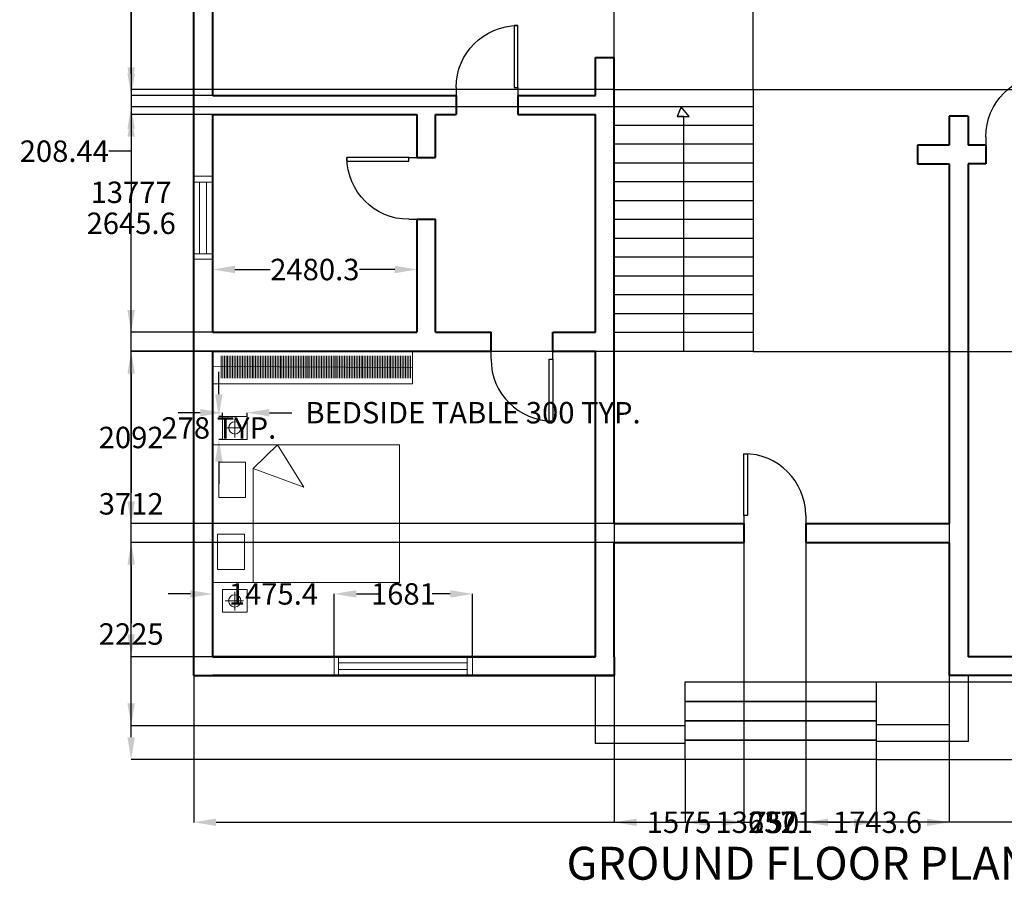
# Model space of a CAD drawing. Units: millimetres. Extents: x 23 to 3809233, y 4 to 290343.
# Tile 1 of 8: x 1896274 to 1908235, y 133276 to 143728. Entities that reach past the tile are written whole.
import ezdxf

# ---------------------------------------------------------------- set-up
doc = ezdxf.new("R2010")
doc.units = ezdxf.units.MM
doc.header["$MEASUREMENT"] = 0
for name, color, linetype, lineweight in [('A-ANNO-DIMS', 2, 'Continuous', 18), ('A-ANNO-TEXT', 7, 'Continuous', 25), ('A-DOOR', 3, 'Continuous', 25), ('A-FLOR-CASE', 8, 'Continuous', 20), ('A-FLOR-STRS', 7, 'Continuous', 25), ('A-FURN', 8, 'Continuous', 18), ('A-FURN-PATT', 252, 'Continuous', 13), ('A-GLAZ', 4, 'Continuous', 18), ('A-WALL', 7, 'Continuous', 40)]:
    doc.layers.add(name, color=color, linetype=linetype, lineweight=lineweight)
doc.styles.get("Standard").update_dxf_attribs({"font": 'arial.ttf'})
doc.dimstyles.get("Standard").update_dxf_attribs({"dimtxt": 260.18, "dimasz": 270.18, "dimexe": 0.18, "dimexo": 0.0625, "dimgap": 0.09, "dimtad": 0, "dimtih": 1, "dimtoh": 1, "dimdec": 0, "dimzin": 0, "dimdsep": 46, "dimtxsty": 'Standard', "dimcen": 0.09, "dimadec": 0, "dimazin": 0, "dimtfac": 1, "dimtdec": 0, "dimtofl": 0, "dimtmove": 0, "dimatfit": 3, "dimfxl": 1, "dimtolj": 1, "dimtzin": 0, "dimarcsym": 0})

# ---------------------------------------------------------------- blocks, each defined once
blk = doc.blocks.new('*U2')
for p, q in [((0, 0), (0, -100)), ((750, 0), (750, -100))]:
    blk.add_line(p, q)
blk.add_lwpolyline([(0, 0), (0, 750), (43.75, 750), (43.75, 0)], close=True)
blk.add_arc((0, 0), 750, 0, 90)
blk = doc.blocks.new('BEDSIDE-TABLE-LAMP')
for p, q in [((150, 247), (150, 23)), ((36, 139), (257, 139))]:
    blk.add_line(p, q)
blk.add_lwpolyline([(0, 275, -0.414214), (3, 278), (297, 278, -0.414214), (300, 275), (300, 3, -0.414214), (297, 0), (3, 0, -0.414214), (0, 3)], format="xyb", close=True)
blk.add_circle((150, 139), 74.8)
blk = doc.blocks.new('*D26')
at = {"layer": 'A-ANNO-DIMS', "color": 0, "lineweight": -2, "transparency": 16777216}
for p, q in [((1898468, 138955), (1898198, 138955)), ((1898738, 138910), (1898738, 138955)), ((1899038, 138910), (1899038, 138955)), ((1899308, 138955), (1899578, 138955))]:
    blk.add_line(p, q, dxfattribs=at)
at = {"layer": 'A-ANNO-DIMS', "color": 0, "transparency": 16777216}
for points in [[(1898468, 139000), (1898468, 138910), (1898738, 138955)], [(1899308, 139000), (1899308, 138910), (1899038, 138955)]]:
    blk.add_solid(points, dxfattribs=at)
at = {"layer": 'Defpoints', "color": 0, "transparency": 16777216}
for p in [(1898738, 138910), (1899038, 138955), (1899038, 138910)]:
    blk.add_point(p, dxfattribs=at)
at = {"layer": 'A-ANNO-DIMS', "color": 0, "transparency": 16777216, "insert": (1901781, 138955), "char_height": 260.18, "attachment_point": 5}
blk.add_mtext('\\A1;BEDSIDE TABLE 300 TYP.', dxfattribs=at)
blk = doc.blocks.new('*D27')
at = {"layer": 'A-ANNO-DIMS', "color": 0, "lineweight": -2, "transparency": 16777216}
for p, q in [((1898693, 139180), (1898693, 139450)), ((1898738, 138910), (1898693, 138910)), ((1898738, 138631), (1898693, 138631)), ((1898693, 138361), (1898693, 138091))]:
    blk.add_line(p, q, dxfattribs=at)
at = {"layer": 'A-ANNO-DIMS', "color": 0, "transparency": 16777216}
for points in [[(1898648, 139180), (1898738, 139180), (1898693, 138910)], [(1898648, 138361), (1898738, 138361), (1898693, 138631)]]:
    blk.add_solid(points, dxfattribs=at)
at = {"layer": 'Defpoints', "color": 0, "transparency": 16777216}
for p in [(1898693, 138910), (1898738, 138910), (1898738, 138631)]:
    blk.add_point(p, dxfattribs=at)
at = {"layer": 'A-ANNO-DIMS', "color": 0, "transparency": 16777216, "insert": (1898693, 138770), "char_height": 260.18, "attachment_point": 5}
blk.add_mtext('\\A1;278 TYP.', dxfattribs=at)
blk = doc.blocks.new('*D48')
at = {"layer": 'A-ANNO-DIMS', "color": 0, "lineweight": -2, "transparency": 16777216}
for p, q in [((1898390, 135763), (1898390, 133980)), ((1912047, 135763), (1912047, 133980)), ((1898660, 133981), (1904741, 133981)), ((1911777, 133981), (1905696, 133981))]:
    blk.add_line(p, q, dxfattribs=at)
at = {"layer": 'A-ANNO-DIMS', "color": 0, "transparency": 16777216}
for points in [[(1898660, 134026), (1898660, 133936), (1898390, 133981)], [(1911777, 134026), (1911777, 133936), (1912047, 133981)]]:
    blk.add_solid(points, dxfattribs=at)
at = {"layer": 'Defpoints', "color": 0, "transparency": 16777216}
for p in [(1898390, 135763), (1912047, 135763), (1912047, 133981)]:
    blk.add_point(p, dxfattribs=at)
at = {"layer": 'A-ANNO-DIMS', "color": 0, "transparency": 16777216, "insert": (1905219, 133981), "char_height": 260.2, "attachment_point": 5}
blk.add_mtext('\\A1;13657', dxfattribs=at)
blk = doc.blocks.new('*D49')
at = {"layer": 'A-ANNO-DIMS', "color": 0, "lineweight": -2, "transparency": 16777216}
for p, q in [((1898389.991383, 148520.288959), (1897627.373883, 148520.288959)), ((1897627.553883, 148250.108959), (1897627.553883, 141764.705112)), ((1897627.553883, 135013.262029), (1897627.553883, 141498.665876)), ((1904356.772229, 134743.082029), (1897627.373883, 134743.082029))]:
    blk.add_line(p, q, dxfattribs=at)
at = {"layer": 'A-ANNO-DIMS', "color": 0, "transparency": 16777216}
for points in [[(1897582.523883, 148250.108959), (1897672.583883, 148250.108959), (1897627.553883, 148520.288959)], [(1897582.523883, 135013.262029), (1897672.583883, 135013.262029), (1897627.553883, 134743.082029)]]:
    blk.add_solid(points, dxfattribs=at)
at = {"layer": 'Defpoints', "color": 0, "transparency": 16777216}
for p in [(1897627.553883, 148520.288959), (1898390.053883, 148520.288959), (1904356.834729, 134743.082029)]:
    blk.add_point(p, dxfattribs=at)
at = {"layer": 'A-ANNO-DIMS', "color": 0, "transparency": 16777216, "insert": (1897627.553883, 141631.685494), "char_height": 260.18, "attachment_point": 5}
blk.add_mtext('\\A1;13777', dxfattribs=at)
blk = doc.blocks.new('*D50')
at = {"layer": 'A-ANNO-DIMS', "color": 0, "lineweight": -2, "transparency": 16777216}
for p, q in [((1898619, 139703), (1897627, 139703)), ((1897628, 139433), (1897628, 137981)), ((1897628, 136262), (1897628, 137715)), ((1898619, 135992), (1897627, 135992))]:
    blk.add_line(p, q, dxfattribs=at)
at = {"layer": 'A-ANNO-DIMS', "color": 0, "transparency": 16777216}
for points in [[(1897583, 139433), (1897673, 139433), (1897628, 139703)], [(1897583, 136262), (1897673, 136262), (1897628, 135992)]]:
    blk.add_solid(points, dxfattribs=at)
at = {"layer": 'Defpoints', "color": 0, "transparency": 16777216}
for p in [(1897628, 139703), (1898619, 139703), (1898619, 135992)]:
    blk.add_point(p, dxfattribs=at)
at = {"layer": 'A-ANNO-DIMS', "color": 0, "transparency": 16777216, "insert": (1897628, 137848), "char_height": 260.2, "attachment_point": 5}
blk.add_mtext('\\A1;3712', dxfattribs=at)
blk = doc.blocks.new('*D51')
at = {"layer": 'A-ANNO-DIMS', "color": 0, "lineweight": -2, "transparency": 16777216}
for p, q in [((1898619, 142578), (1897627, 142578)), ((1897628, 142307), (1897628, 141388)), ((1897628, 140202), (1897628, 141122)), ((1898619, 139932), (1897627, 139932))]:
    blk.add_line(p, q, dxfattribs=at)
at = {"layer": 'A-ANNO-DIMS', "color": 0, "transparency": 16777216}
for points in [[(1897583, 142307), (1897673, 142307), (1897628, 142578)], [(1897583, 140202), (1897673, 140202), (1897628, 139932)]]:
    blk.add_solid(points, dxfattribs=at)
at = {"layer": 'Defpoints', "color": 0, "transparency": 16777216}
for p in [(1897628, 142578), (1898619, 142578), (1898619, 139932)]:
    blk.add_point(p, dxfattribs=at)
at = {"layer": 'A-ANNO-DIMS', "color": 0, "transparency": 16777216, "insert": (1897628, 141255), "char_height": 260.2, "attachment_point": 5}
blk.add_mtext('\\A1;2645.6', dxfattribs=at)
blk = doc.blocks.new('*D52')
at = {"layer": 'A-ANNO-DIMS', "color": 0, "lineweight": -2, "transparency": 16777216}
for p, q in [((1898619, 148292), (1897627, 148292)), ((1897628, 148022), (1897628, 145682)), ((1897628, 143076), (1897628, 145416)), ((1898619, 142806), (1897627, 142806))]:
    blk.add_line(p, q, dxfattribs=at)
at = {"layer": 'A-ANNO-DIMS', "color": 0, "transparency": 16777216}
for points in [[(1897583, 148022), (1897673, 148022), (1897628, 148292)], [(1897583, 143076), (1897673, 143076), (1897628, 142806)]]:
    blk.add_solid(points, dxfattribs=at)
at = {"layer": 'Defpoints', "color": 0, "transparency": 16777216}
for p in [(1897628, 148292), (1898619, 148292), (1898619, 142806)]:
    blk.add_point(p, dxfattribs=at)
at = {"layer": 'A-ANNO-DIMS', "color": 0, "transparency": 16777216, "insert": (1897628, 145549), "char_height": 260.2, "attachment_point": 5}
blk.add_mtext('\\A1;5485', dxfattribs=at)
blk = doc.blocks.new('*D56')
at = {"layer": 'A-ANNO-DIMS', "color": 0, "lineweight": -2, "transparency": 16777216}
for p, q in [((1898619, 139932), (1898619, 140695)), ((1898889, 140694), (1899316, 140694)), ((1900829, 140694), (1900401, 140694)), ((1901099, 139932), (1901099, 140695))]:
    blk.add_line(p, q, dxfattribs=at)
at = {"layer": 'A-ANNO-DIMS', "color": 0, "transparency": 16777216}
for points in [[(1898889, 140740), (1898889, 140649), (1898619, 140694)], [(1900829, 140740), (1900829, 140649), (1901099, 140694)]]:
    blk.add_solid(points, dxfattribs=at)
at = {"layer": 'Defpoints', "color": 0, "transparency": 16777216}
for p in [(1901099, 140694), (1898619, 139932), (1901099, 139932)]:
    blk.add_point(p, dxfattribs=at)
at = {"layer": 'A-ANNO-DIMS', "color": 0, "transparency": 16777216, "insert": (1899859, 140694), "char_height": 260.2, "attachment_point": 5}
blk.add_mtext('\\A1;2480.3', dxfattribs=at)
blk = doc.blocks.new('*D67')
at = {"layer": 'A-ANNO-DIMS', "color": 0, "lineweight": -2, "transparency": 16777216}
for p, q in [((1898348, 136754), (1898078, 136754)), ((1898619, 135992), (1898619, 136754)), ((1900094, 135992), (1900094, 136754)), ((1900364, 136754), (1900634, 136754))]:
    blk.add_line(p, q, dxfattribs=at)
at = {"layer": 'A-ANNO-DIMS', "color": 0, "transparency": 16777216}
for points in [[(1898348, 136799), (1898348, 136709), (1898619, 136754)], [(1900364, 136799), (1900364, 136709), (1900094, 136754)]]:
    blk.add_solid(points, dxfattribs=at)
at = {"layer": 'Defpoints', "color": 0, "transparency": 16777216}
for p in [(1900094, 136754), (1898619, 135992), (1900094, 135992)]:
    blk.add_point(p, dxfattribs=at)
at = {"layer": 'A-ANNO-DIMS', "color": 0, "transparency": 16777216, "insert": (1899356, 136754), "char_height": 260.2, "attachment_point": 5}
blk.add_mtext('\\A1;1475.4', dxfattribs=at)
blk = doc.blocks.new('*D68')
at = {"layer": 'A-ANNO-DIMS', "color": 0, "lineweight": -2, "transparency": 16777216}
for p, q in [((1900094, 135992), (1900094, 136754)), ((1900364, 136754), (1900583, 136754)), ((1901505, 136754), (1901286, 136754)), ((1901775, 135992), (1901775, 136754))]:
    blk.add_line(p, q, dxfattribs=at)
at = {"layer": 'A-ANNO-DIMS', "color": 0, "transparency": 16777216}
for points in [[(1900364, 136799), (1900364, 136709), (1900094, 136754)], [(1901505, 136799), (1901505, 136709), (1901775, 136754)]]:
    blk.add_solid(points, dxfattribs=at)
at = {"layer": 'Defpoints', "color": 0, "transparency": 16777216}
for p in [(1901775, 136754), (1900094, 135992), (1901775, 135992)]:
    blk.add_point(p, dxfattribs=at)
at = {"layer": 'A-ANNO-DIMS', "color": 0, "transparency": 16777216, "insert": (1900935, 136754), "char_height": 260.2, "attachment_point": 5}
blk.add_mtext('\\A1;1681', dxfattribs=at)
blk = doc.blocks.new('*D70')
at = {"layer": 'A-ANNO-DIMS', "color": 0, "lineweight": -2, "transparency": 16777216}
for p, q in [((1903497, 142880), (1903497, 149283)), ((1903767, 149283), (1903964, 149283)), ((1904913, 149283), (1904716, 149283)), ((1905183, 142880), (1905183, 149283))]:
    blk.add_line(p, q, dxfattribs=at)
at = {"layer": 'A-ANNO-DIMS', "color": 0, "transparency": 16777216}
for points in [[(1903767, 149328), (1903767, 149238), (1903497, 149283)], [(1904913, 149328), (1904913, 149238), (1905183, 149283)]]:
    blk.add_solid(points, dxfattribs=at)
at = {"layer": 'Defpoints', "color": 0, "transparency": 16777216}
for p in [(1905183, 149283), (1903497, 142880), (1905183, 142880)]:
    blk.add_point(p, dxfattribs=at)
at = {"layer": 'A-ANNO-DIMS', "color": 0, "transparency": 16777216, "insert": (1904340, 149283), "char_height": 260.2, "attachment_point": 5}
blk.add_mtext('\\A1;1686', dxfattribs=at)
blk = doc.blocks.new('*D71')
at = {"layer": 'A-ANNO-DIMS', "color": 0, "lineweight": -2, "transparency": 16777216}
for p, q in [((1905183, 142880), (1912810, 142880)), ((1912810, 142610), (1912810, 141423)), ((1912810, 139970), (1912810, 141157)), ((1905183, 139700), (1912810, 139700))]:
    blk.add_line(p, q, dxfattribs=at)
at = {"layer": 'A-ANNO-DIMS', "color": 0, "transparency": 16777216}
for points in [[(1912765, 142610), (1912855, 142610), (1912810, 142880)], [(1912765, 139970), (1912855, 139970), (1912810, 139700)]]:
    blk.add_solid(points, dxfattribs=at)
at = {"layer": 'Defpoints', "color": 0, "transparency": 16777216}
for p in [(1905183, 142880), (1912810, 142880), (1905183, 139700)]:
    blk.add_point(p, dxfattribs=at)
at = {"layer": 'A-ANNO-DIMS', "color": 0, "transparency": 16777216, "insert": (1912810, 141290), "char_height": 260.2, "attachment_point": 5}
blk.add_mtext('\\A1;3180', dxfattribs=at)
blk = doc.blocks.new('*D72')
at = {"layer": 'A-ANNO-DIMS', "color": 0, "lineweight": -2, "transparency": 16777216}
for p, q in [((1897628, 143150), (1897628, 143420)), ((1903497, 142880), (1897627, 142880)), ((1903497, 142671), (1897627, 142671)), ((1897628, 142401), (1897628, 142131)), ((1897628, 142131), (1897357, 142131))]:
    blk.add_line(p, q, dxfattribs=at)
at = {"layer": 'A-ANNO-DIMS', "color": 0, "transparency": 16777216}
for points in [[(1897583, 143150), (1897673, 143150), (1897628, 142880)], [(1897583, 142401), (1897673, 142401), (1897628, 142671)]]:
    blk.add_solid(points, dxfattribs=at)
at = {"layer": 'Defpoints', "color": 0, "transparency": 16777216}
for p in [(1903497, 142880), (1897628, 142671), (1903497, 142671)]:
    blk.add_point(p, dxfattribs=at)
at = {"layer": 'A-ANNO-DIMS', "color": 0, "transparency": 16777216, "insert": (1896816, 142131), "char_height": 260.2, "attachment_point": 5}
blk.add_mtext('\\A1;208.44', dxfattribs=at)
blk = doc.blocks.new('*D73')
at = {"layer": 'A-ANNO-DIMS', "color": 0, "lineweight": -2, "transparency": 16777216}
for p, q in [((1903497, 139700), (1897627, 139700)), ((1897628, 139429), (1897628, 138787)), ((1897628, 137878), (1897628, 138521)), ((1903497, 137608), (1897627, 137608))]:
    blk.add_line(p, q, dxfattribs=at)
at = {"layer": 'A-ANNO-DIMS', "color": 0, "transparency": 16777216}
for points in [[(1897583, 139429), (1897673, 139429), (1897628, 139700)], [(1897583, 137878), (1897673, 137878), (1897628, 137608)]]:
    blk.add_solid(points, dxfattribs=at)
at = {"layer": 'Defpoints', "color": 0, "transparency": 16777216}
for p in [(1897628, 139700), (1903497, 139700), (1903497, 137608)]:
    blk.add_point(p, dxfattribs=at)
at = {"layer": 'A-ANNO-DIMS', "color": 0, "transparency": 16777216, "insert": (1897628, 138654), "char_height": 260.2, "attachment_point": 5}
blk.add_mtext('\\A1;2092', dxfattribs=at)
blk = doc.blocks.new('*D74')
at = {"layer": 'A-ANNO-DIMS', "color": 0, "lineweight": -2, "transparency": 16777216}
for p, q in [((1903497, 137608), (1903497, 133980)), ((1905072, 137608), (1905072, 133980)), ((1903767, 133981), (1903907, 133981)), ((1904802, 133981), (1904662, 133981))]:
    blk.add_line(p, q, dxfattribs=at)
at = {"layer": 'A-ANNO-DIMS', "color": 0, "transparency": 16777216}
for points in [[(1903767, 134026), (1903767, 133936), (1903497, 133981)], [(1904802, 134026), (1904802, 133936), (1905072, 133981)]]:
    blk.add_solid(points, dxfattribs=at)
at = {"layer": 'Defpoints', "color": 0, "transparency": 16777216}
for p in [(1903497, 137608), (1905072, 137608), (1905072, 133981)]:
    blk.add_point(p, dxfattribs=at)
at = {"layer": 'A-ANNO-DIMS', "color": 0, "transparency": 16777216, "insert": (1904285, 133981), "char_height": 260.2, "attachment_point": 5}
blk.add_mtext('\\A1;1575', dxfattribs=at)
blk = doc.blocks.new('*D75')
at = {"layer": 'A-ANNO-DIMS', "color": 0, "lineweight": -2, "transparency": 16777216}
for p, q in [((1905072.156133, 137607.670665), (1905072.156133, 133980.402029)), ((1905822.156133, 137607.670665), (1905822.156133, 133980.402029)), ((1904801.976133, 133980.582029), (1904531.796133, 133980.582029)), ((1906092.336133, 133980.582029), (1906362.516133, 133980.582029))]:
    blk.add_line(p, q, dxfattribs=at)
at = {"layer": 'A-ANNO-DIMS', "color": 0, "transparency": 16777216}
for points in [[(1904801.976133, 134025.612029), (1904801.976133, 133935.552029), (1905072.156133, 133980.582029)], [(1906092.336133, 134025.612029), (1906092.336133, 133935.552029), (1905822.156133, 133980.582029)]]:
    blk.add_solid(points, dxfattribs=at)
at = {"layer": 'Defpoints', "color": 0, "transparency": 16777216}
for p in [(1905072.156133, 137607.733165), (1905822.156133, 137607.733165), (1905822.156133, 133980.582029)]:
    blk.add_point(p, dxfattribs=at)
at = {"layer": 'A-ANNO-DIMS', "color": 0, "transparency": 16777216, "insert": (1905447.156133, 133980.582029), "char_height": 260.18, "attachment_point": 5}
blk.add_mtext('\\A1;750', dxfattribs=at)
blk = doc.blocks.new('*D76')
at = {"layer": 'A-ANNO-DIMS', "color": 0, "lineweight": -2, "transparency": 16777216}
for p, q in [((1905822, 137608), (1905822, 133980)), ((1907566, 137608), (1907566, 133980)), ((1906092, 133981), (1906166, 133981)), ((1907296, 133981), (1907222, 133981))]:
    blk.add_line(p, q, dxfattribs=at)
at = {"layer": 'A-ANNO-DIMS', "color": 0, "transparency": 16777216}
for points in [[(1906092, 134026), (1906092, 133936), (1905822, 133981)], [(1907296, 134026), (1907296, 133936), (1907566, 133981)]]:
    blk.add_solid(points, dxfattribs=at)
at = {"layer": 'Defpoints', "color": 0, "transparency": 16777216}
for p in [(1905822, 137608), (1907566, 137608), (1907566, 133981)]:
    blk.add_point(p, dxfattribs=at)
at = {"layer": 'A-ANNO-DIMS', "color": 0, "transparency": 16777216, "insert": (1906694, 133981), "char_height": 260.2, "attachment_point": 5}
blk.add_mtext('\\A1;1743.6', dxfattribs=at)
blk = doc.blocks.new('*D77')
at = {"layer": 'A-ANNO-DIMS', "color": 0, "lineweight": -2, "transparency": 16777216}
for p, q in [((1903497, 137379), (1897627, 137379)), ((1897628, 137109), (1897628, 136400)), ((1897628, 135424), (1897628, 136134)), ((1903497, 135154), (1897627, 135154))]:
    blk.add_line(p, q, dxfattribs=at)
at = {"layer": 'A-ANNO-DIMS', "color": 0, "transparency": 16777216}
for points in [[(1897583, 137109), (1897673, 137109), (1897628, 137379)], [(1897583, 135424), (1897673, 135424), (1897628, 135154)]]:
    blk.add_solid(points, dxfattribs=at)
at = {"layer": 'Defpoints', "color": 0, "transparency": 16777216}
for p in [(1903497, 137379), (1897628, 135154), (1903497, 135154)]:
    blk.add_point(p, dxfattribs=at)
at = {"layer": 'A-ANNO-DIMS', "color": 0, "transparency": 16777216, "insert": (1897628, 136267), "char_height": 260.2, "attachment_point": 5}
blk.add_mtext('\\A1;2225', dxfattribs=at)
blk = doc.blocks.new('*D78')
at = {"layer": 'A-ANNO-DIMS', "color": 0, "lineweight": -2, "transparency": 16777216}
for p, q in [((1904357, 134743), (1904357, 133980)), ((1906678, 134743), (1906678, 133980)), ((1904627, 133981), (1905152, 133981)), ((1906408, 133981), (1905883, 133981))]:
    blk.add_line(p, q, dxfattribs=at)
at = {"layer": 'A-ANNO-DIMS', "color": 0, "transparency": 16777216}
for points in [[(1904627, 134026), (1904627, 133936), (1904357, 133981)], [(1906408, 134026), (1906408, 133936), (1906678, 133981)]]:
    blk.add_solid(points, dxfattribs=at)
at = {"layer": 'Defpoints', "color": 0, "transparency": 16777216}
for p in [(1904357, 134743), (1906678, 134743), (1906678, 133981)]:
    blk.add_point(p, dxfattribs=at)
at = {"layer": 'A-ANNO-DIMS', "color": 0, "transparency": 16777216, "insert": (1905517, 133981), "char_height": 260.2, "attachment_point": 5}
blk.add_mtext('\\A1;2321', dxfattribs=at)
blk = doc.blocks.new('*D79')
at = {"layer": 'A-ANNO-DIMS', "color": 0, "lineweight": -2, "transparency": 16777216}
for p, q in [((1906678, 135685), (1912810, 135685)), ((1912810, 135414), (1912810, 135347)), ((1912810, 135013), (1912810, 135081)), ((1906678, 134743), (1912810, 134743))]:
    blk.add_line(p, q, dxfattribs=at)
at = {"layer": 'A-ANNO-DIMS', "color": 0, "transparency": 16777216}
for points in [[(1912765, 135414), (1912855, 135414), (1912810, 135685)], [(1912765, 135013), (1912855, 135013), (1912810, 134743)]]:
    blk.add_solid(points, dxfattribs=at)
at = {"layer": 'Defpoints', "color": 0, "transparency": 16777216}
for p in [(1906678, 135685), (1912810, 135685), (1906678, 134743)]:
    blk.add_point(p, dxfattribs=at)
at = {"layer": 'A-ANNO-DIMS', "color": 0, "transparency": 16777216, "insert": (1912810, 135214), "char_height": 260.2, "attachment_point": 5}
blk.add_mtext('\\A1;941.5', dxfattribs=at)

msp = doc.modelspace()

# ---------------------------------------------------------------- hatches: boundary and pattern name
at = {"layer": 'A-FURN-PATT'}
h = msp.add_hatch(dxfattribs=at)
h.set_pattern_fill('ANSI31', color=256, scale=160, angle=45, style=0)
h.paths.add_polyline_path([(1898717.182, 139373.351), (1901027.182, 139373.351), (1901027.182, 139645.723), (1898717.182, 139645.723)])

# ---------------------------------------------------------------- linework, layer by layer
at = {"layer": 'A-FLOR-CASE'}
for p, q in [((1901047.38, 139304.455), (1901047.38, 139703.398)), ((1898618.654, 139516.636), (1901047.38, 139503.927)), ((1898618.654, 139304.455), (1901047.38, 139304.455))]:
    msp.add_line(p, q, dxfattribs=at)
at = {"layer": 'A-FLOR-STRS'}
for p, q in [((1903497.165, 142879.905), (1905183.132, 142879.905)), ((1905183.132, 142879.905), (1905183.132, 139699.662)), ((1905183.132, 142671.462), (1903497.165, 142671.462)), ((1904309.134, 142671.462), (1904261.487, 142552.081)), ((1904405.226, 142552.081), (1904309.134, 142671.462)), ((1904340.149, 142552.081), (1904261.487, 142552.081)), ((1904261.487, 142552.081), (1904405.226, 142552.081)), ((1904340.149, 139699.662), (1904340.149, 142552.081)), ((1905183.132, 142442.862), (1903497.165, 142442.862)), ((1905183.132, 142214.262), (1903497.165, 142214.262)), ((1905183.132, 141985.662), (1903497.165, 141985.662)), ((1905183.132, 141757.062), (1903497.165, 141757.062)), ((1905183.132, 141528.462), (1903497.165, 141528.462)), ((1905183.132, 141299.862), (1903497.165, 141299.862)), ((1905183.132, 141071.262), (1903497.165, 141071.262)), ((1905183.132, 140842.662), (1903497.165, 140842.662)), ((1905183.132, 140614.062), (1903497.165, 140614.062)), ((1905183.132, 140385.462), (1903497.165, 140385.462)), ((1905183.132, 140156.862), (1903497.165, 140156.862)), ((1905183.132, 139928.262), (1903497.165, 139928.262)), ((1905183.132, 139699.662), (1903497.165, 139699.662)), ((1903264.191, 135763.089), (1903264.191, 134940.968)), ((1903497.165, 135763.089), (1903497.165, 135154.307)), ((1907565.715, 135763.089), (1907565.715, 135165.93)), ((1907794.315, 135763.089), (1907794.315, 135141.164)), ((1907565.715, 135165.93), (1906677.88, 135165.93)), ((1903497.165, 135154.307), (1904356.835, 135154.307)), ((1907794.315, 135141.164), (1907794.315, 134976.318)), ((1903264.191, 134940.968), (1904356.835, 134940.968)), ((1907794.315, 134960.55), (1906677.88, 134960.55)), ((1907794.315, 134976.318), (1907794.315, 134960.55))]:
    msp.add_line(p, q, dxfattribs=at)
for points in [[(1904356.835, 135684.558), (1906677.88, 135684.558), (1906677.88, 135449.189), (1904356.835, 135449.189)], [(1904356.835, 135449.189), (1906677.88, 135449.189), (1906677.88, 135213.82), (1904356.835, 135213.82)], [(1904356.835, 135213.82), (1906677.88, 135213.82), (1906677.88, 134978.451), (1904356.835, 134978.451)], [(1904356.835, 134978.451), (1906677.88, 134978.451), (1906677.88, 134743.082), (1904356.835, 134743.082)]]:
    msp.add_lwpolyline(points, close=True, dxfattribs=at)
at = {"layer": 'A-FURN'}
for p, q in [((1899108.354, 138275.646), (1899405.743, 138562.91)), ((1899405.743, 138562.91), (1899725.502, 138051.702)), ((1899108.354, 136894.058), (1899108.354, 138275.646)), ((1899725.502, 138051.702), (1899108.354, 138275.646))]:
    msp.add_line(p, q, dxfattribs=at)
for points in [[(1898618.654, 138559.91, -0.414213562), (1898621.654, 138562.91), (1900883.921, 138562.91, -0.414213562), (1900886.921, 138559.91), (1900886.921, 136897.058, -0.414213562), (1900883.921, 136894.058), (1898621.654, 136894.058, -0.414213562), (1898618.654, 136897.058)], [(1898691.027, 138350.809, -0.414213562), (1898694.027, 138353.809), (1899014.311, 138353.809, -0.414213562), (1899017.311, 138350.809), (1899017.311, 137927.473, -0.414213562), (1899014.311, 137924.473), (1898694.027, 137924.473, -0.414213562), (1898691.027, 137927.473)], [(1898678.077, 137476.62, -0.414213562), (1898681.077, 137479.62), (1899001.361, 137479.62, -0.414213562), (1899004.361, 137476.62), (1899004.361, 137053.284, -0.414213562), (1899001.361, 137050.284), (1898681.077, 137050.284, -0.414213562), (1898678.077, 137053.284)]]:
    msp.add_lwpolyline(points, format="xyb", close=True, dxfattribs=at)
at = {"layer": 'A-GLAZ'}
for p, q in [((1898390.054, 141829.043), (1898618.654, 141829.043)), ((1898618.654, 141755.477), (1898390.054, 141755.477)), ((1898458.737, 141755.477), (1898458.737, 140882.957)), ((1898543.893, 141755.477), (1898543.893, 140882.957)), ((1898390.054, 140882.957), (1898618.654, 140882.957)), ((1898390.054, 140818.049), (1898618.654, 140818.049)), ((1900094.099, 135991.689), (1900094.099, 135763.089)), ((1900147.958, 135991.689), (1900147.958, 135763.089)), ((1900147.958, 135916.628), (1901710.175, 135916.628)), ((1901710.175, 135991.689), (1901710.175, 135763.089)), ((1901710.175, 135877.389), (1901710.175, 135877.389)), ((1901774.996, 135991.689), (1901774.996, 135763.089)), ((1900147.958, 135836.003), (1901710.175, 135836.003)), ((1900943.61, 135763.089), (1900943.61, 135763.089))]:
    msp.add_line(p, q, dxfattribs=at)
at = {"layer": 'A-WALL'}
for p, q in [((1898390.054, 135763.089), (1898390.054, 148520.289)), ((1898618.654, 142806.221), (1898618.654, 148291.689)), ((1903268.565, 142806.221), (1903268.565, 143267.727)), ((1903268.565, 143267.727), (1903497.165, 143267.727)), ((1903497.165, 137607.733), (1903497.165, 143267.727)), ((1898618.654, 142806.221), (1901575.786, 142806.221)), ((1901575.786, 142806.221), (1901575.786, 142577.621)), ((1902325.786, 142806.221), (1902325.786, 142577.621)), ((1902325.786, 142806.221), (1903268.565, 142806.221)), ((1898618.654, 142577.621), (1901098.98, 142577.621)), ((1898618.654, 139931.998), (1898618.654, 142577.621)), ((1901098.98, 142577.621), (1901098.98, 142054.184)), ((1901326.466, 142577.621), (1901575.786, 142577.621)), ((1901326.466, 142054.184), (1901326.466, 142577.621)), ((1902325.786, 142577.621), (1903268.565, 142577.621)), ((1903268.565, 139931.998), (1903268.565, 142577.621)), ((1903497.165, 137607.733), (1903497.165, 142577.621)), ((1907565.715, 142554.593), (1907565.715, 142204.876)), ((1907794.315, 142554.593), (1907565.715, 142554.593)), ((1907794.315, 142554.593), (1907794.315, 142204.876)), ((1907565.715, 142204.876), (1907180.661, 142204.876)), ((1907180.661, 142204.876), (1907180.661, 141976.276)), ((1908009.428, 142204.876), (1907794.315, 142204.876)), ((1908009.428, 142204.876), (1908009.428, 142020.244)), ((1901098.98, 142054.184), (1901326.466, 142054.184)), ((1908009.428, 142020.244), (1908009.428, 141976.276)), ((1907180.661, 141976.276), (1907565.715, 141976.276)), ((1907565.715, 141976.276), (1907565.715, 137607.733)), ((1907794.315, 141976.276), (1907794.315, 135991.689)), ((1908009.428, 141976.276), (1907794.315, 141976.276)), ((1901098.98, 141304.184), (1901326.466, 141304.184)), ((1901098.98, 141304.184), (1901098.98, 139931.998)), ((1901326.466, 139931.998), (1901326.466, 141304.184)), ((1898618.654, 139931.998), (1901098.98, 139931.998)), ((1901326.466, 139931.998), (1901999.547, 139931.998)), ((1901999.547, 139703.398), (1901999.547, 139931.998)), ((1902749.547, 139703.398), (1902749.547, 139931.998)), ((1902749.547, 139931.998), (1903268.565, 139931.998)), ((1898618.654, 135991.689), (1898618.654, 139703.398)), ((1898618.654, 139703.398), (1901999.547, 139703.398)), ((1902749.547, 139703.398), (1903268.565, 139703.398)), ((1903268.565, 135991.689), (1903268.565, 139703.398)), ((1903497.165, 137607.733), (1905072.156, 137607.733)), ((1905072.156, 137607.733), (1905072.156, 137379.133)), ((1905822.156, 137607.733), (1905822.156, 137379.133)), ((1905822.156, 137607.733), (1907565.715, 137607.733)), ((1903497.165, 135991.689), (1903497.165, 137379.133)), ((1903497.165, 135991.689), (1903497.165, 137379.133)), ((1903497.165, 137379.133), (1905072.156, 137379.133)), ((1905822.156, 137379.133), (1907565.715, 137379.133)), ((1907565.715, 137379.133), (1907565.715, 135991.689)), ((1898618.654, 135991.689), (1903268.565, 135991.689)), ((1903268.565, 135991.689), (1898618.654, 135991.689)), ((1903497.165, 135991.689), (1903497.165, 135763.089)), ((1907565.715, 135991.689), (1907565.715, 135763.089)), ((1908469.731, 135991.689), (1907794.315, 135991.689)), ((1898390.054, 135763.089), (1903497.165, 135763.089)), ((1903497.165, 135763.089), (1898618.654, 135763.089)), ((1908469.731, 135763.089), (1907565.715, 135763.089))]:
    msp.add_line(p, q, dxfattribs=at)

# ---------------------------------------------------------------- block references
at = {"layer": 'A-DOOR', "xscale": -1}
for p in [(1902325.786, 142906.221), (1908759.428, 142304.876)]:
    msp.add_blockref('*U2', p, dxfattribs=at)
at = {"layer": 'A-DOOR', "xscale": -1, "rotation": 90}
msp.add_blockref('*U2', (1900998.98, 142054.184), dxfattribs=at)
at = {"layer": 'A-DOOR', "rotation": 180}
msp.add_blockref('*U2', (1902749.547, 139603.398), dxfattribs=at)
at = {"layer": 'A-DOOR'}
msp.add_blockref('*U2', (1905072.156, 137707.225), dxfattribs=at)
at = {"layer": 'A-FURN'}
for p in [(1898737.988, 138631.22), (1898735.436, 136530.927)]:
    msp.add_blockref('BEDSIDE-TABLE-LAMP', p, dxfattribs=at)

# ---------------------------------------------------------------- texts
at = {"layer": 'A-ANNO-TEXT', "insert": (1902916.406, 133683.241), "char_height": 400, "attachment_point": 1}
msp.add_mtext_dynamic_manual_height_columns('GROUND FLOOR PLAN', width=8410.77875, gutter_width=1, heights=[0], dxfattribs=at)

# ---------------------------------------------------------------- dimensions: what is measured, and where the dimension line sits
at = {"layer": 'A-ANNO-DIMS'}
for base, p1, p2, override, picture, middle in [((1905183.132, 149282.789), (1903497.165, 142879.905), (1905183.132, 142879.905), {"dimdec": 0, "dimlfac": 1, "dimrnd": 0, "dimzin": 0, "dimdsep": 46, "dimlunit": 2}, '*D70', (1904340.149, 149282.789)), ((1901098.98, 140694.498), (1898618.654, 139931.998), (1901098.98, 139931.998), {"dimdec": 1, "dimlfac": 1, "dimrnd": 0, "dimzin": 0, "dimdsep": 46, "dimlunit": 2}, '*D56', (1899858.817, 140694.498)), ((1905072.156, 133980.582), (1903497.165, 137607.733), (1905072.156, 137607.733), {"dimdec": 0, "dimlfac": 1, "dimrnd": 0, "dimzin": 0, "dimdsep": 46, "dimlunit": 2}, '*D74', (1904284.661, 133980.582)), ((1905822.156, 133980.582), (1905072.156, 137607.733), (1905822.156, 137607.733), {"dimdec": 0, "dimlfac": 1, "dimrnd": 0, "dimzin": 0, "dimdsep": 46, "dimlunit": 2}, '*D75', (1905447.156, 133980.582)), ((1907565.715, 133980.582), (1905822.156, 137607.733), (1907565.715, 137607.733), {"dimdec": 1, "dimlfac": 1, "dimrnd": 0, "dimzin": 0, "dimdsep": 46, "dimlunit": 2}, '*D76', (1906693.936, 133980.582)), ((1900094.099, 136754.189), (1898618.654, 135991.689), (1900094.099, 135991.689), {"dimdec": 1, "dimlfac": 1, "dimrnd": 0, "dimzin": 0, "dimdsep": 46, "dimlunit": 2}, '*D67', (1899356.376, 136754.189)), ((1901774.996, 136754.189), (1900094.099, 135991.689), (1901774.996, 135991.689), {"dimdec": 0, "dimlfac": 1, "dimrnd": 0, "dimzin": 0, "dimdsep": 46, "dimlunit": 2}, '*D68', (1900934.548, 136754.189)), ((1912047.254, 133980.582), (1898390.054, 135763.089), (1912047.254, 135763.089), {"dimdec": 0, "dimlfac": 1, "dimrnd": 0, "dimzin": 0, "dimdsep": 46, "dimlunit": 2}, '*D48', (1905218.654, 133980.582)), ((1906677.88, 133980.582), (1904356.835, 134743.082), (1906677.88, 134743.082), {"dimdec": 0, "dimlfac": 1, "dimrnd": 0, "dimzin": 0, "dimdsep": 46, "dimlunit": 2}, '*D78', (1905517.357, 133980.582))]:
    dim = msp.add_linear_dim(base=base, p1=p1, p2=p2, dimstyle='Standard', override=override, dxfattribs=at)
    dim.commit()
    dim.dimension.update_dxf_attribs({"geometry": picture, "text_midpoint": middle})
for base, p1, p2, override, picture, middle in [((1897627.554, 148520.289), (1904356.835, 134743.082), (1898390.054, 148520.289), {"dimdec": 0, "dimlfac": 1, "dimrnd": 0, "dimzin": 0, "dimdsep": 46, "dimlunit": 2}, '*D49', (1897627.554, 141631.685)), ((1897627.554, 148291.689), (1898618.654, 142806.221), (1898618.654, 148291.689), {"dimdec": 0, "dimlfac": 1, "dimrnd": 0, "dimzin": 0, "dimdsep": 46, "dimlunit": 2}, '*D52', (1897627.554, 145548.955)), ((1897627.554, 142671.462), (1903497.165, 142879.905), (1903497.165, 142671.462), {"dimdec": 2, "dimlfac": 1, "dimrnd": 0, "dimzin": 0, "dimdsep": 46, "dimlunit": 2}, '*D72', (1896815.538, 142131.102)), ((1912809.754, 142879.905), (1905183.132, 139699.662), (1905183.132, 142879.905), {"dimdec": 0, "dimlfac": 1, "dimrnd": 0, "dimzin": 0, "dimdsep": 46, "dimlunit": 2}, '*D71', (1912809.754, 141289.783)), ((1897627.554, 142577.621), (1898618.654, 139931.998), (1898618.654, 142577.621), {"dimdec": 1, "dimlfac": 1, "dimrnd": 0, "dimzin": 0, "dimdsep": 46, "dimlunit": 2}, '*D51', (1897627.554, 141254.809)), ((1897627.554, 139703.398), (1898618.654, 135991.689), (1898618.654, 139703.398), {"dimdec": 0, "dimlfac": 1, "dimrnd": 0, "dimzin": 0, "dimdsep": 46, "dimlunit": 2}, '*D50', (1897627.554, 137847.543)), ((1897627.554, 139699.662), (1903497.165, 137607.733), (1903497.165, 139699.662), {"dimdec": 0, "dimlfac": 1, "dimrnd": 0, "dimzin": 0, "dimdsep": 46, "dimlunit": 2}, '*D73', (1897627.554, 138653.697)), ((1897627.554, 135154.307), (1903497.165, 137379.133), (1903497.165, 135154.307), {"dimdec": 0, "dimlfac": 1, "dimrnd": 0, "dimzin": 0, "dimdsep": 46, "dimlunit": 2}, '*D77', (1897627.554, 136266.72)), ((1912809.754, 135684.558), (1906677.88, 134743.082), (1906677.88, 135684.558), {"dimdec": 1, "dimlfac": 1, "dimrnd": 0, "dimzin": 0, "dimdsep": 46, "dimlunit": 2}, '*D79', (1912809.754, 135213.82))]:
    dim = msp.add_linear_dim(base=base, p1=p1, p2=p2, angle=90, dimstyle='Standard', override=override, dxfattribs=at)
    dim.commit()
    dim.dimension.update_dxf_attribs({"geometry": picture, "text_midpoint": middle})
dim = msp.add_linear_dim(base=(1899037.775, 138954.591), p1=(1898737.988, 138909.623), p2=(1899037.775, 138909.623), text='BEDSIDE TABLE <> TYP.', dimstyle='Standard', override={"dimdec": 0, "dimlfac": 1, "dimrnd": 0, "dimzin": 0, "dimdsep": 46, "dimlunit": 2}, dxfattribs=at)
dim.commit()
dim.dimension.update_dxf_attribs({"geometry": '*D26', "text_midpoint": (1901781.324, 138954.591)})
dim = msp.add_linear_dim(base=(1898693.02, 138909.623), p1=(1898737.988, 138631.22), p2=(1898737.988, 138909.623), angle=90, text='<> TYP.', dimstyle='Standard', override={"dimdec": 0, "dimlfac": 1, "dimrnd": 0, "dimzin": 0, "dimdsep": 46, "dimlunit": 2}, dxfattribs=at)
dim.commit()
dim.dimension.update_dxf_attribs({"geometry": '*D27', "text_midpoint": (1898693.02, 138770.421)})

doc.saveas('drawing.dxf')
